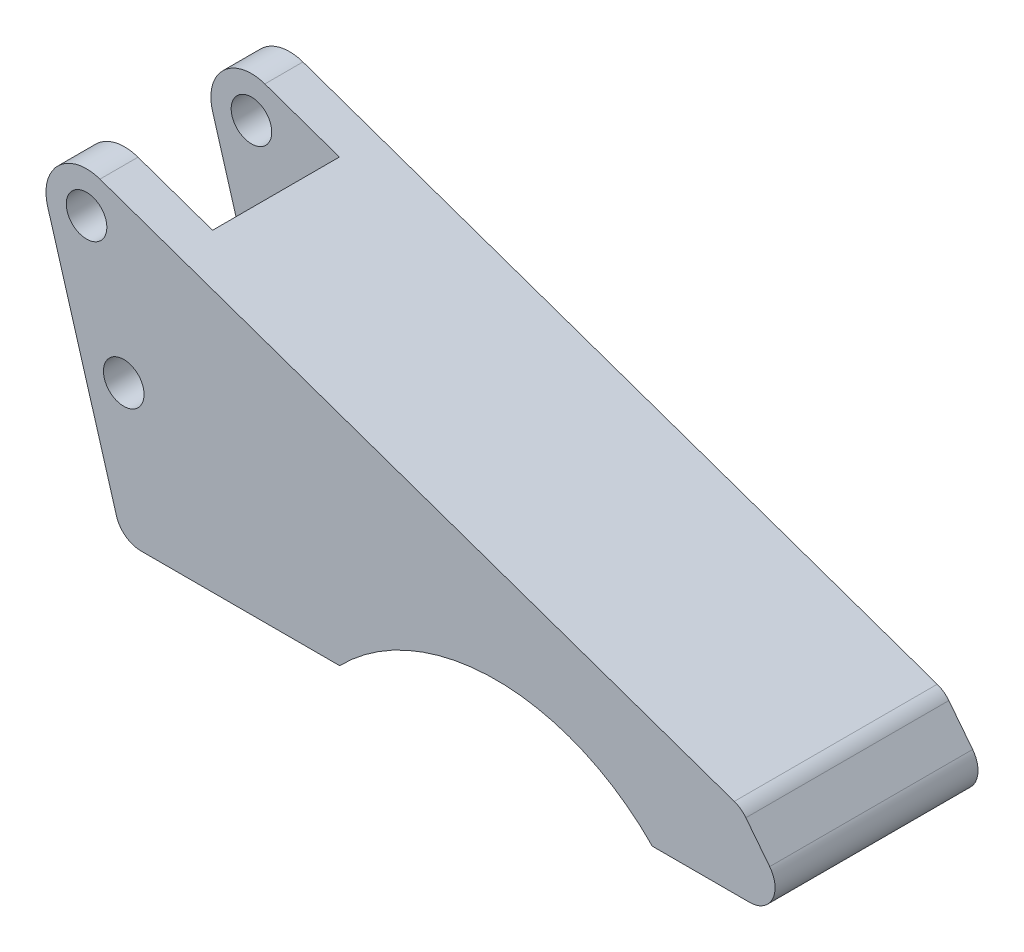
from build123d import *

# Parameters (mm, degrees)
JAW_PROFILE_SKETCH_R        = 4
JAW_PLATE_40MM_DEPTH        = 20
CLEVIS_SLOT_25MM_DEPTH      = 107.52257834
CLEVIS_SLOT_25MM_DEPTH_BACK = 107.52257834
CLEVIS_SLOT_SKETCH_W        = 50
CLEVIS_SLOT_SKETCH_H        = 25


with BuildPart() as part:
    # Jaw Profile Sketch → Jaw Plate 40mm (new, symmetric)
    with BuildSketch(Plane.XY):
        with BuildLine():
            Line((-39.194156399, 0), (0, 0))
            ThreePointArc((0, 0), (30.805843601, 13), (61.611687203, 0))
            Line((61.611687203, 0), (80.805843601, 0))
            ThreePointArc((80.805843601, 0), (85.299901044, 2.808323085), (84.745652382, 8.07862092))
            Line((84.745652382, 8.07862092), (80.057169629, 14.07862092))
            ThreePointArc((80.057169629, 14.07862092), (79.030253505, 15.063872091), (77.767360848, 15.71990466))
            Line((77.767360848, 15.71990466), (-47.244156399, 59.421847456))
            ThreePointArc((-47.244156399, 59.421847456), (-55.398946719, 57.665436802), (-57.55764481, 49.607794087))
            Line((-57.55764481, 49.607794087), (-43.990086656, 3.586121305))
            ThreePointArc((-43.990086656, 3.586121305), (-42.188368025, 0.995665256), (-39.194156399, 0))
        make_face()
        with Locations((-49.884156399, 51.87)):
            Circle(JAW_PROFILE_SKETCH_R, mode=Mode.SUBTRACT)
        with Locations((-42.554156399, 27)):
            Circle(JAW_PROFILE_SKETCH_R, mode=Mode.SUBTRACT)
    extrude(amount=JAW_PLATE_40MM_DEPTH, both=True)

    # Clevis Slot Sketch → Clevis Slot 25mm (cut, two sides: drawn at the far end of the back side and taken through both)
    with BuildSketch(Plane.XZ.offset(-CLEVIS_SLOT_25MM_DEPTH_BACK)):
        with Locations((-57.55764481, 0)):
            Rectangle(CLEVIS_SLOT_SKETCH_W, CLEVIS_SLOT_SKETCH_H)
    extrude(amount=CLEVIS_SLOT_25MM_DEPTH + CLEVIS_SLOT_25MM_DEPTH_BACK, mode=Mode.SUBTRACT)


solid = part.part
